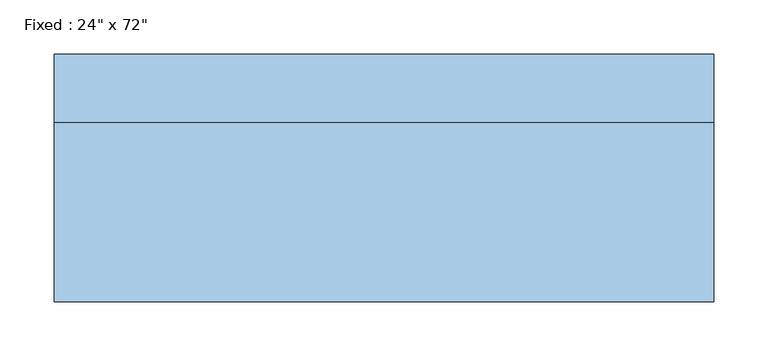
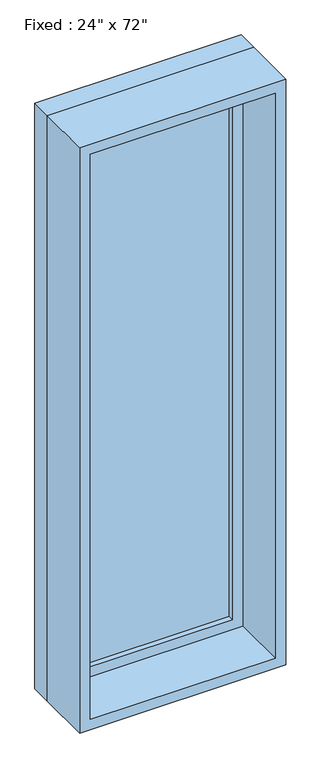
"""IFC4 building model written with IfcOpenShell, lengths in millimetres: window geometry."""

from ifc_helpers import new_model, si_unit, frame, origin, place, context, project, spatial, polyline, outline, extrude, source, transform, mapped, element, save


def window_fc882ab3(model_context):
    return source(origin(), model_context, "Body", "SweptSolid", [
        extrude(outline(polyline([(203.2, 66.675), (-279.4, 66.675), (-279.4, 79.375), (203.2, 79.375), (203.2, 66.675)])), frame((0.0, 0.0, 368.3), z_axis=(0.0, 0.0, 1.0), x_axis=(1.0, 0.0, 0.0)), (0.0, 0.0, 1.0), 1701.8),
        extrude(outline(polyline([(2114.55, -323.85), (323.85, -323.85), (323.85, 247.65), (2114.55, 247.65), (2114.55, -323.85)]), holes=[polyline([(2070.1, -279.4), (2070.1, 203.2), (368.3, 203.2), (368.3, -279.4), (2070.1, -279.4)])]), frame((0.0, 50.8, 0.0), z_axis=(0.0, 1.0, 0.0), x_axis=(0.0, 0.0, 1.0)), (0.0, 0.0, 1.0), 44.45),
        extrude(outline(polyline([(2133.6, -342.9), (304.8, -342.9), (304.8, 266.7), (2133.6, 266.7), (2133.6, -342.9)]), holes=[polyline([(2101.85, -311.15), (2101.85, 234.95), (336.55, 234.95), (336.55, -311.15), (2101.85, -311.15)])]), frame((0.0, -114.3, 0.0), z_axis=(0.0, 1.0, 0.0), x_axis=(0.0, 0.0, 1.0)), (0.0, 0.0, 1.0), 165.1),
        extrude(outline(polyline([(2133.6, 266.7), (2133.6, -342.9), (304.8, -342.9), (304.8, 266.7), (2133.6, 266.7)]), holes=[polyline([(2114.55, 247.65), (323.85, 247.65), (323.85, -323.85), (2114.55, -323.85), (2114.55, 247.65)])]), frame((0.0, 50.8, 0.0), z_axis=(0.0, 1.0, 0.0), x_axis=(0.0, 0.0, 1.0)), (0.0, 0.0, 1.0), 63.5),
    ])


if __name__ == "__main__":
    model = new_model("IFC4")
    model_context = context("Model", 3, world=origin())
    ifc_project = project(units=[si_unit("LENGTHUNIT", "METRE", prefix="MILLI")], contexts=[model_context])
    site = spatial("IfcSite", under=ifc_project)
    building = spatial("IfcBuilding", under=site)
    placement = place(None, origin())
    window_shape = window_fc882ab3(model_context)
    element("IfcWindow", 1, ObjectType="Fixed : 24\" x 72\"", at=placement, inside=building, context=model_context, shape_type="MappedRepresentation", body=[
        mapped(window_shape, transform((0.0, 0.0, 0.0), x_axis=(1.0, 0.0, 0.0), y_axis=(0.0, 1.0, 0.0), z_axis=(0.0, 0.0, 1.0))),
    ])
    save(model, "model.ifc")

# Revit data of these elements
# Type "Fixed : 24\" x 72\""
#   Type Mark = "7"
#   Construction Type Id = "GSP4R"
#   Assembly Code = "B2020100"
#   Analytic Construction = "1/8 in Pilkington single glazing"
#   Visual Light Transmittance = 0.9
#   Solar Heat Gain Coefficient = 0.78
#   Heat Transfer Coefficient (U) = 0.6496 BTU/(h·ft²·°F)
#   Height = 6' - 0"
#   Default Sill Height = 1' - 0"
#   Width = 2' - 0"
#   Window Inset = 0' - 0 3/4"
#   Define Thermal Properties by = 1
#   Glass Pane Material = Glass
#   Sash Material = Sash
#   Wall Closure = (empty or 0)
# Element 1 (IfcWindow, "Fixed : 24\" x 72\"")
#   Materials on its faces: "Sash", "Glass"
# Materials
#   "Glass": class "Glass", colour RGB 0 128 192, transparency 0.75, Description = "Soda Lime Glass", Cost = 0
#   "Sash": class "Wood", colour RGB 224 178 126, transparency 0
